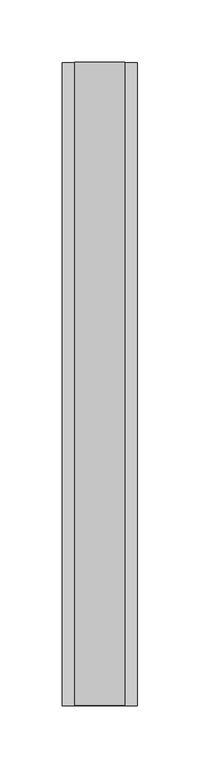
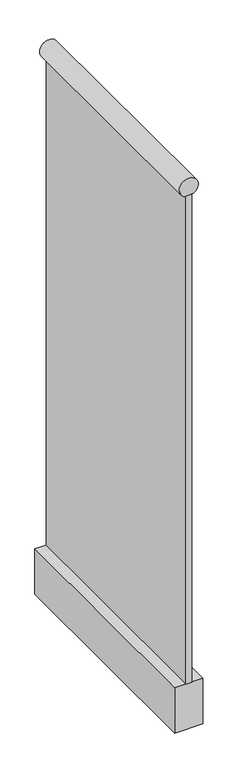
"""IFC4 building model written with IfcOpenShell, lengths in millimetres: railing geometry."""

from ifc_helpers import new_model, si_unit, point, frame, frame_2d, origin, place, context, project, spatial, polyline, circle_curve, trimmed, segment, composite_curve, outline, extrude, source, transform, mapped, element, save


def railing_926c3c2b(model_context):
    return source(origin(), model_context, "Body", "SweptSolid", [
        extrude(outline(composite_curve([segment(trimmed(circle_curve(frame_2d((5015.3205081, -1533.8712297)), 20.0), [point((4998.0, -1523.8712297))], [point((4998.0, -1543.8712297))], False, "CARTESIAN"), True, "CONTINUOUS"), segment(polyline([(4998.0, -1543.8712297), (4998.0, -1523.8712297)]), True, "CONTINUOUS")], self_intersect=False)), frame((0.0, -7637.0014262, 0.0), z_axis=(0.0, 1.0, 0.0), x_axis=(0.0, 0.0, 1.0)), (0.0, 0.0, 1.0), 515.0),
        extrude(outline(polyline([(-1527.8712297, -7637.0014262), (-1539.8712297, -7637.0014262), (-1539.8712297, -7122.0014262), (-1527.8712297, -7122.0014262), (-1527.8712297, -7637.0014262)])), frame((0.0, 0.0, 3900.0), z_axis=(0.0, 0.0, 1.0), x_axis=(1.0, 0.0, 0.0)), (0.0, 0.0, 1.0), 1098.0),
        extrude(outline(polyline([(-1503.8712297, -7637.0014262), (-1563.8712297, -7637.0014262), (-1563.8712297, -7122.0014262), (-1503.8712297, -7122.0014262), (-1503.8712297, -7637.0014262)])), frame((0.0, 0.0, 3798.0), z_axis=(0.0, 0.0, 1.0), x_axis=(1.0, 0.0, 0.0)), (0.0, 0.0, 1.0), 102.0),
    ])


if __name__ == "__main__":
    model = new_model("IFC4")
    model_context = context("Model", 3, world=origin())
    ifc_project = project(units=[si_unit("LENGTHUNIT", "METRE", prefix="MILLI")], contexts=[model_context])
    site = spatial("IfcSite", under=ifc_project)
    building = spatial("IfcBuilding", under=site)
    placement = place(None, origin())
    railing_shape = railing_926c3c2b(model_context)
    element("IfcRailing", 1, at=placement, inside=building, context=model_context, shape_type="MappedRepresentation", body=[
        mapped(railing_shape, transform((0.0, 0.0, 0.0), x_axis=(1.0, 0.0, 0.0), y_axis=(0.0, 1.0, 0.0), z_axis=(0.0, 0.0, 1.0))),
    ])
    save(model, "model.ifc")

# Revit data of these elements
# Element 1 (IfcRailing)
#   Materials on its faces: "Metal - Aluminum"
# Materials
#   "Metal - Aluminum": colour RGB 247 247 247, transparency 0, Cost = 0
